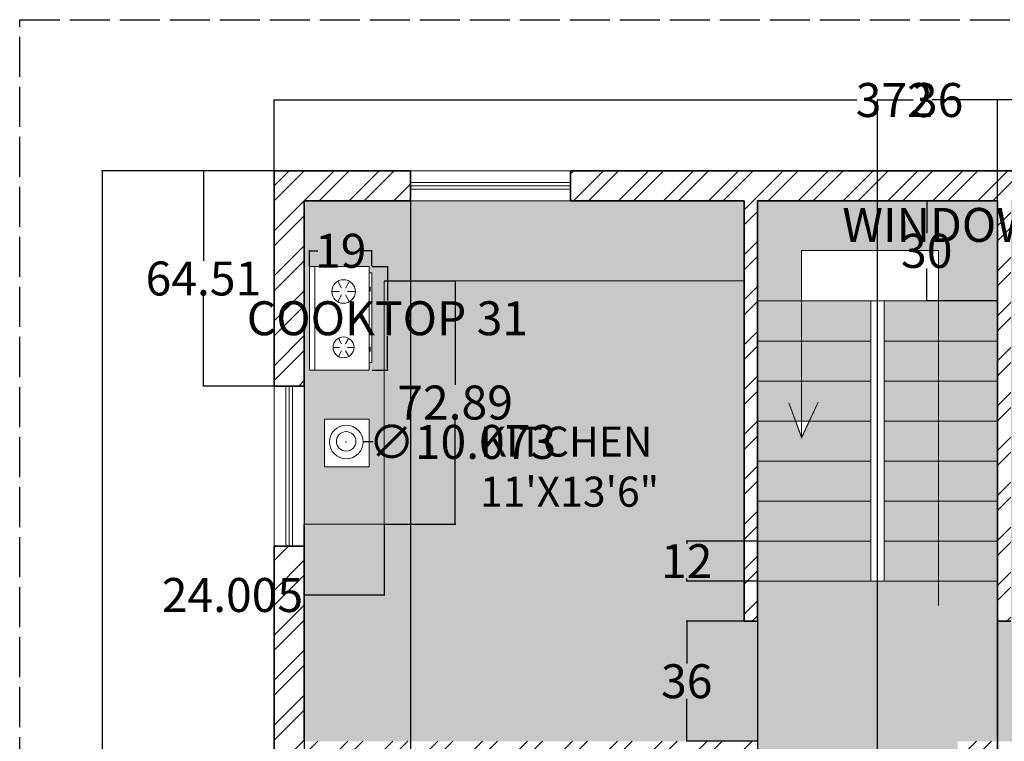
# Model space of a CAD drawing. Units: inches. Extents: x 1410 to 1959, y 5441 to 5968.
# Tile 2 of 5: x 1410 to 1705, y 5751 to 5968. Entities that reach past the tile are written whole.
import ezdxf

# ---------------------------------------------------------------- set-up
doc = ezdxf.new("R2010")
doc.units = ezdxf.units.IN
doc.linetypes.add('ACAD_ISO02W100', pattern=[15, 12, -3])
doc.layers.get('Defpoints').update_dxf_attribs({"linetype": 'ACAD_ISO02W100'})
for name, color, linetype, lineweight in [('A-ANNO-DIMS', 2, 'Continuous', 18), ('A-ANNO-SYMB', 7, 'Continuous', 18), ('A-AREA-IDEN', 7, 'Continuous', 18), ('A-EQPM', 15, 'Continuous', 15), ('A-FLOR-CABT', 15, 'Continuous', 18), ('A-FLOR-FIXT', 9, 'Continuous', 18), ('A-FLOR-STRS', 7, 'Continuous', 18), ('A-WALL', 7, 'Continuous', 35), ('A-WALL-PATT', 8, 'Continuous', 13), ('WINDOW', 160, 'Continuous', 13)]:
    doc.layers.add(name, color=color, linetype=linetype, lineweight=lineweight)
for name, color, linetype, lineweight, true_color in [('A-FLOR-CABT-PATT', 165, 'Continuous', 9, 0x5e67af), ('A-FLOR-PATT', 9, 'Continuous', 9, 0xafd9aa), ('A-FLOR-STRS-PATT', 254, 'Continuous', 9, 0xddb3d4), ('FURN3D', 229, 'Continuous', 5, 0x4a3f41)]:
    doc.layers.add(name, color=color, linetype=linetype, lineweight=lineweight, true_color=true_color)
doc.styles.get("Standard").update_dxf_attribs({"font": 'arial.ttf'})
doc.dimstyles.get("Standard").update_dxf_attribs({"dimtxt": 10.18, "dimasz": 0.18, "dimexe": 0.18, "dimexo": 0.0625, "dimgap": 0.09, "dimtad": 0, "dimtih": 1, "dimtoh": 1, "dimdec": 0, "dimzin": 0, "dimdsep": 46, "dimlunit": 3, "dimtxsty": 'Standard', "dimcen": 0.09, "dimadec": 0, "dimazin": 0, "dimtfac": 1, "dimtdec": 0, "dimtofl": 0, "dimtmove": 0, "dimatfit": 3, "dimfxl": 1, "dimtolj": 1, "dimtzin": 0, "dimarcsym": 0})

# ---------------------------------------------------------------- blocks, each defined once
blk = doc.blocks.new('A$C21540130')
at = {"layer": 'FURN3D'}
for p, q in [((1.57, 0), (1.57, 31.11)), ((9.61, 25.31), (8.63, 27.01)), ((10.79, 25.31), (11.77, 27.01)), ((9.02, 24.29, -27.54), (7.06, 24.29, -27.54)), ((11.38, 24.29, -27.54), (13.34, 24.29, -27.54)), ((9.61, 23.27), (8.63, 21.57)), ((10.79, 23.27), (11.77, 21.57)), ((9.61, 8.56), (8.43, 10.6)), ((10.79, 8.56), (11.97, 10.6)), ((9.02, 7.54), (6.67, 7.54)), ((9.61, 6.52), (8.43, 4.48)), ((10.79, 6.52), (11.97, 4.48)), ((11.38, 7.54), (13.73, 7.54))]:
    blk.add_line(p, q, dxfattribs=at)
for points in [[(0, 0), (0, 31.11), (17.9, 31.11), (17.9, 0)], [(18.68, 1.96), (18.68, 28.83), (17.9, 28.83), (17.9, 1.96)]]:
    blk.add_lwpolyline(points, close=True, dxfattribs=at)
for centre, radius in [((10.2, 24.29), 3.14), ((10.2, 7.54), 3.53)]:
    blk.add_circle(centre, radius, dxfattribs=at)
for points in [[(17.9, 24.03), (18.29, 24.03), (17.9, 25.6), (18.29, 25.6)], [(17.9, 6.05), (18.29, 6.05), (17.9, 7.62), (18.29, 7.62)]]:
    blk.add_solid(points, dxfattribs=at)
blk = doc.blocks.new('WIN-48IN')
for p, q in [((48, 9), (0, 9)), ((0, 5.5), (48, 5.5)), ((0, 4.5), (48, 4.5)), ((0, 3.5), (48, 3.5)), ((0, 0), (48, 0))]:
    blk.add_line(p, q)
blk = doc.blocks.new('*D10')
at = {"layer": 'A-ANNO-DIMS', "color": 0, "lineweight": -2, "transparency": 16777216}
for p, q in [((1769.1, 5913.3), (1769.1, 5905.99)), ((1817.1, 5913.3), (1817.1, 5905.99)), ((1769.1, 5906.17), (1768.92, 5906.17)), ((1816.92, 5906.17), (1769.28, 5906.17))]:
    blk.add_line(p, q, dxfattribs=at)
at = {"layer": 'A-ANNO-DIMS', "color": 0, "transparency": 16777216}
for points in [[(1769.28, 5906.2), (1769.28, 5906.14), (1769.1, 5906.17)], [(1816.92, 5906.2), (1816.92, 5906.14), (1817.1, 5906.17)]]:
    blk.add_solid(points, dxfattribs=at)
at = {"layer": 'Defpoints', "color": 0, "transparency": 16777216}
for p in [(1769.1, 5913.37), (1817.1, 5913.37), (1769.1, 5906.17)]:
    blk.add_point(p, dxfattribs=at)
at = {"layer": 'A-ANNO-DIMS', "color": 0, "transparency": 16777216, "insert": (1710.67, 5906.17), "char_height": 10.18, "attachment_point": 5}
blk.add_mtext('\\A1;WINDOW 48 TYP.', dxfattribs=at)
blk = doc.blocks.new('*D20')
at = {"layer": 'A-ANNO-DIMS', "color": 0, "lineweight": -2, "transparency": 16777216}
for p, q in [((1515.44, 5893.75), (1520.23, 5893.75)), ((1520.05, 5893.57), (1520.05, 5883.56)), ((1520.05, 5862.82), (1520.05, 5872.83)), ((1515.44, 5862.64), (1520.23, 5862.64))]:
    blk.add_line(p, q, dxfattribs=at)
at = {"layer": 'A-ANNO-DIMS', "color": 0, "transparency": 16777216}
for points in [[(1520.02, 5893.57), (1520.08, 5893.57), (1520.05, 5893.75)], [(1520.02, 5862.82), (1520.08, 5862.82), (1520.05, 5862.64)]]:
    blk.add_solid(points, dxfattribs=at)
at = {"layer": 'Defpoints', "color": 0, "transparency": 16777216}
for p in [(1515.38, 5893.75), (1515.38, 5862.64), (1520.05, 5862.64)]:
    blk.add_point(p, dxfattribs=at)
at = {"layer": 'A-ANNO-DIMS', "color": 0, "transparency": 16777216, "insert": (1520.05, 5878.19), "char_height": 10.18, "attachment_point": 5}
blk.add_mtext('\\A1;COOKTOP 31', dxfattribs=at)
blk = doc.blocks.new('*D21')
at = {"layer": 'A-ANNO-DIMS', "color": 0, "lineweight": -2, "transparency": 16777216}
for p, q in [((1496.7, 5893.81), (1496.7, 5898.59)), ((1496.88, 5898.41), (1499.13, 5898.41)), ((1515.2, 5898.41), (1512.95, 5898.41)), ((1515.38, 5893.81), (1515.38, 5898.59))]:
    blk.add_line(p, q, dxfattribs=at)
at = {"layer": 'A-ANNO-DIMS', "color": 0, "transparency": 16777216}
for points in [[(1496.88, 5898.44), (1496.88, 5898.38), (1496.7, 5898.41)], [(1515.2, 5898.44), (1515.2, 5898.38), (1515.38, 5898.41)]]:
    blk.add_solid(points, dxfattribs=at)
at = {"layer": 'Defpoints', "color": 0, "transparency": 16777216}
for p in [(1515.38, 5898.41), (1496.7, 5893.75), (1515.38, 5893.75)]:
    blk.add_point(p, dxfattribs=at)
at = {"layer": 'A-ANNO-DIMS', "color": 0, "transparency": 16777216, "insert": (1506.04, 5898.41), "char_height": 10.18, "attachment_point": 5}
blk.add_mtext('\\A1;19', dxfattribs=at)
blk = doc.blocks.new('*D24')
at = {"layer": 'A-ANNO-DIMS', "color": 0, "lineweight": -2, "transparency": 16777216}
for p, q in [((1486.09, 5922.43), (1486.09, 5943.8)), ((1486.27, 5943.62), (1660.81, 5943.62)), ((1857.91, 5943.62), (1683.37, 5943.62)), ((1858.09, 5922.43), (1858.09, 5943.8))]:
    blk.add_line(p, q, dxfattribs=at)
at = {"layer": 'A-ANNO-DIMS', "color": 0, "transparency": 16777216}
for points in [[(1486.27, 5943.65), (1486.27, 5943.59), (1486.09, 5943.62)], [(1857.91, 5943.65), (1857.91, 5943.59), (1858.09, 5943.62)]]:
    blk.add_solid(points, dxfattribs=at)
at = {"layer": 'Defpoints', "color": 0, "transparency": 16777216}
for p in [(1858.09, 5943.62), (1486.09, 5922.37), (1858.09, 5922.37)]:
    blk.add_point(p, dxfattribs=at)
at = {"layer": 'A-ANNO-DIMS', "color": 0, "transparency": 16777216, "insert": (1672.09, 5943.62), "char_height": 10.18, "attachment_point": 5}
blk.add_mtext('\\A1;372', dxfattribs=at)
blk = doc.blocks.new('*D25')
at = {"layer": 'A-ANNO-DIMS', "color": 0, "lineweight": -2, "transparency": 16777216}
for p, q in [((1486.03, 5922.37), (1434.27, 5922.37)), ((1434.45, 5922.19), (1434.45, 5729.66)), ((1434.45, 5526.55), (1434.45, 5719.07)), ((1703.03, 5526.37), (1434.27, 5526.37))]:
    blk.add_line(p, q, dxfattribs=at)
at = {"layer": 'A-ANNO-DIMS', "color": 0, "transparency": 16777216}
for points in [[(1434.42, 5922.19), (1434.48, 5922.19), (1434.45, 5922.37)], [(1434.42, 5526.55), (1434.48, 5526.55), (1434.45, 5526.37)]]:
    blk.add_solid(points, dxfattribs=at)
at = {"layer": 'Defpoints', "color": 0, "transparency": 16777216}
for p in [(1434.45, 5922.37), (1486.09, 5922.37), (1703.09, 5526.37)]:
    blk.add_point(p, dxfattribs=at)
at = {"layer": 'A-ANNO-DIMS', "color": 0, "transparency": 16777216, "insert": (1434.45, 5724.37), "char_height": 10.18, "attachment_point": 5}
blk.add_mtext('\\A1;396', dxfattribs=at)
blk = doc.blocks.new('*D27')
at = {"layer": 'A-ANNO-DIMS', "color": 0, "lineweight": -2, "transparency": 16777216}
for p, q in [((1495.09, 5913.3), (1495.09, 5478.87)), ((1527, 5913.3), (1527, 5478.87)), ((1495.27, 5479.05), (1526.82, 5479.05)), ((1527, 5479.05), (1527.18, 5479.05))]:
    blk.add_line(p, q, dxfattribs=at)
at = {"layer": 'A-ANNO-DIMS', "color": 0, "transparency": 16777216}
for points in [[(1495.27, 5479.08), (1495.27, 5479.02), (1495.09, 5479.05)], [(1526.82, 5479.08), (1526.82, 5479.02), (1527, 5479.05)]]:
    blk.add_solid(points, dxfattribs=at)
at = {"layer": 'Defpoints', "color": 0, "transparency": 16777216}
for p in [(1495.09, 5913.37), (1527, 5913.37), (1527, 5479.05)]:
    blk.add_point(p, dxfattribs=at)
at = {"layer": 'A-ANNO-DIMS', "color": 0, "transparency": 16777216, "insert": (1548.43, 5479.05), "char_height": 10.18, "attachment_point": 5}
blk.add_mtext('\\A1;31.905', dxfattribs=at)
blk = doc.blocks.new('*D29')
at = {"layer": 'A-ANNO-DIMS', "color": 0, "lineweight": -2, "transparency": 16777216}
for p, q in [((1486.03, 5922.37), (1464.66, 5922.36)), ((1464.84, 5922.18), (1464.85, 5895.4)), ((1464.85, 5858.03), (1464.85, 5884.82)), ((1486.04, 5857.86), (1464.67, 5857.85))]:
    blk.add_line(p, q, dxfattribs=at)
at = {"layer": 'A-ANNO-DIMS', "color": 0, "transparency": 16777216}
for points in [[(1464.87, 5922.18), (1464.81, 5922.18), (1464.84, 5922.36)], [(1464.88, 5858.03), (1464.82, 5858.03), (1464.85, 5857.85)]]:
    blk.add_solid(points, dxfattribs=at)
at = {"layer": 'Defpoints', "color": 0, "transparency": 16777216}
for p in [(1464.84, 5922.36), (1486.09, 5922.37), (1486.1, 5857.86)]:
    blk.add_point(p, dxfattribs=at)
at = {"layer": 'A-ANNO-DIMS', "color": 0, "transparency": 16777216, "insert": (1464.85, 5890.11), "char_height": 10.18, "attachment_point": 5}
blk.add_mtext('\\A1;64.51', dxfattribs=at)
blk = doc.blocks.new('*D34')
at = {"layer": 'A-ANNO-DIMS', "color": 0, "lineweight": -2, "transparency": 16777216}
for p, q in [((1631.09, 5787.3), (1631.09, 5478.87)), ((1703.09, 5787.3), (1703.09, 5478.87)), ((1631.27, 5479.05), (1659.81, 5479.05)), ((1702.91, 5479.05), (1674.38, 5479.05))]:
    blk.add_line(p, q, dxfattribs=at)
at = {"layer": 'A-ANNO-DIMS', "color": 0, "transparency": 16777216}
for points in [[(1631.27, 5479.08), (1631.27, 5479.02), (1631.09, 5479.05)], [(1702.91, 5479.08), (1702.91, 5479.02), (1703.09, 5479.05)]]:
    blk.add_solid(points, dxfattribs=at)
at = {"layer": 'Defpoints', "color": 0, "transparency": 16777216}
for p in [(1631.09, 5787.37), (1703.09, 5787.37), (1703.09, 5479.05)]:
    blk.add_point(p, dxfattribs=at)
at = {"layer": 'A-ANNO-DIMS', "color": 0, "transparency": 16777216, "insert": (1667.09, 5479.05), "char_height": 10.18, "attachment_point": 5}
blk.add_mtext('\\A1;72', dxfattribs=at)
blk = doc.blocks.new('*D35')
at = {"layer": 'A-ANNO-DIMS', "color": 0, "lineweight": -2, "transparency": 16777216}
for p, q in [((1631.03, 5787.37), (1609.66, 5787.37)), ((1609.84, 5787.19), (1609.84, 5774.66)), ((1609.84, 5751.55), (1609.84, 5764.07)), ((1631.03, 5751.37), (1609.66, 5751.37))]:
    blk.add_line(p, q, dxfattribs=at)
at = {"layer": 'A-ANNO-DIMS', "color": 0, "transparency": 16777216}
for points in [[(1609.81, 5787.19), (1609.87, 5787.19), (1609.84, 5787.37)], [(1609.81, 5751.55), (1609.87, 5751.55), (1609.84, 5751.37)]]:
    blk.add_solid(points, dxfattribs=at)
at = {"layer": 'Defpoints', "color": 0, "transparency": 16777216}
for p in [(1609.84, 5787.37), (1631.09, 5787.37), (1631.09, 5751.37)]:
    blk.add_point(p, dxfattribs=at)
at = {"layer": 'A-ANNO-DIMS', "color": 0, "transparency": 16777216, "insert": (1609.84, 5769.37), "char_height": 10.18, "attachment_point": 5}
blk.add_mtext('\\A1;36', dxfattribs=at)
blk = doc.blocks.new('*D37')
at = {"layer": 'A-ANNO-DIMS', "color": 0, "lineweight": -2, "transparency": 16777216}
for p, q in [((1667.09, 5594.43), (1667.09, 5943.8)), ((1667.27, 5943.62), (1677.72, 5943.62)), ((1702.91, 5943.62), (1692.47, 5943.62)), ((1703.09, 5558.43), (1703.09, 5943.8))]:
    blk.add_line(p, q, dxfattribs=at)
at = {"layer": 'A-ANNO-DIMS', "color": 0, "transparency": 16777216}
for points in [[(1667.27, 5943.65), (1667.27, 5943.59), (1667.09, 5943.62)], [(1702.91, 5943.65), (1702.91, 5943.59), (1703.09, 5943.62)]]:
    blk.add_solid(points, dxfattribs=at)
at = {"layer": 'Defpoints', "color": 0, "transparency": 16777216}
for p in [(1703.09, 5943.62), (1667.09, 5594.37), (1703.09, 5558.37)]:
    blk.add_point(p, dxfattribs=at)
at = {"layer": 'A-ANNO-DIMS', "color": 0, "transparency": 16777216, "insert": (1685.09, 5943.62), "char_height": 10.18, "attachment_point": 5}
blk.add_mtext('\\A1;36', dxfattribs=at)
blk = doc.blocks.new('*D49')
at = {"layer": 'A-ANNO-DIMS', "color": 0, "lineweight": -2, "transparency": 16777216}
for p, q in [((1495.09, 5816.41), (1495.09, 5795.04)), ((1519.1, 5816.41), (1519.1, 5795.04)), ((1495.09, 5795.22), (1494.91, 5795.22)), ((1518.92, 5795.22), (1495.27, 5795.22))]:
    blk.add_line(p, q, dxfattribs=at)
at = {"layer": 'A-ANNO-DIMS', "color": 0, "transparency": 16777216}
for points in [[(1495.27, 5795.25), (1495.27, 5795.19), (1495.09, 5795.22)], [(1518.92, 5795.25), (1518.92, 5795.19), (1519.1, 5795.22)]]:
    blk.add_solid(points, dxfattribs=at)
at = {"layer": 'Defpoints', "color": 0, "transparency": 16777216}
for p in [(1495.09, 5816.47), (1519.1, 5816.47), (1495.09, 5795.22)]:
    blk.add_point(p, dxfattribs=at)
at = {"layer": 'A-ANNO-DIMS', "color": 0, "transparency": 16777216, "insert": (1473.57, 5795.22), "char_height": 10.18, "attachment_point": 5}
blk.add_mtext('\\A1;24.005', dxfattribs=at)
blk = doc.blocks.new('*D50')
at = {"layer": 'A-ANNO-DIMS', "color": 0, "lineweight": -2, "transparency": 16777216}
for p, q in [((1519.16, 5889.37), (1540.53, 5889.37)), ((1540.35, 5889.19), (1540.35, 5858.21)), ((1540.35, 5816.65), (1540.35, 5847.63)), ((1519.16, 5816.47), (1540.53, 5816.47))]:
    blk.add_line(p, q, dxfattribs=at)
at = {"layer": 'A-ANNO-DIMS', "color": 0, "transparency": 16777216}
for points in [[(1540.32, 5889.19), (1540.38, 5889.19), (1540.35, 5889.37)], [(1540.32, 5816.65), (1540.38, 5816.65), (1540.35, 5816.47)]]:
    blk.add_solid(points, dxfattribs=at)
at = {"layer": 'Defpoints', "color": 0, "transparency": 16777216}
for p in [(1519.1, 5889.37), (1519.1, 5816.47), (1540.35, 5816.47)]:
    blk.add_point(p, dxfattribs=at)
at = {"layer": 'A-ANNO-DIMS', "color": 0, "transparency": 16777216, "insert": (1540.35, 5852.92), "char_height": 10.18, "attachment_point": 5}
blk.add_mtext('\\A1;72.89', dxfattribs=at)
blk = doc.blocks.new('*D51')
at = {"layer": 'A-ANNO-DIMS', "color": 0, "lineweight": -2, "transparency": 16777216}
for p, q in [((1631.03, 5811.37), (1609.66, 5811.37)), ((1609.84, 5811.19), (1609.84, 5810.57)), ((1631.03, 5799.37), (1609.66, 5799.37)), ((1609.84, 5799.55), (1609.84, 5800.17))]:
    blk.add_line(p, q, dxfattribs=at)
at = {"layer": 'A-ANNO-DIMS', "color": 0, "transparency": 16777216}
for points in [[(1609.81, 5811.19), (1609.87, 5811.19), (1609.84, 5811.37)], [(1609.81, 5799.55), (1609.87, 5799.55), (1609.84, 5799.37)]]:
    blk.add_solid(points, dxfattribs=at)
at = {"layer": 'Defpoints', "color": 0, "transparency": 16777216}
for p in [(1609.84, 5811.37), (1631.09, 5811.37), (1631.09, 5799.37)]:
    blk.add_point(p, dxfattribs=at)
at = {"layer": 'A-ANNO-DIMS', "color": 0, "transparency": 16777216, "insert": (1609.84, 5805.37), "char_height": 10.18, "attachment_point": 5}
blk.add_mtext('\\A1;12', dxfattribs=at)
blk = doc.blocks.new('*D52')
at = {"layer": 'A-ANNO-DIMS', "color": 0, "lineweight": -2, "transparency": 16777216}
for p, q in [((1703.03, 5913.37), (1681.66, 5913.37)), ((1681.84, 5913.19), (1681.84, 5903.66)), ((1681.84, 5883.55), (1681.84, 5893.07)), ((1703.03, 5883.37), (1681.66, 5883.37))]:
    blk.add_line(p, q, dxfattribs=at)
at = {"layer": 'A-ANNO-DIMS', "color": 0, "transparency": 16777216}
for points in [[(1681.81, 5913.19), (1681.87, 5913.19), (1681.84, 5913.37)], [(1681.81, 5883.55), (1681.87, 5883.55), (1681.84, 5883.37)]]:
    blk.add_solid(points, dxfattribs=at)
at = {"layer": 'Defpoints', "color": 0, "transparency": 16777216}
for p in [(1681.84, 5913.37), (1703.09, 5913.37), (1703.09, 5883.37)]:
    blk.add_point(p, dxfattribs=at)
at = {"layer": 'A-ANNO-DIMS', "color": 0, "transparency": 16777216, "insert": (1681.84, 5898.37), "char_height": 10.18, "attachment_point": 5}
blk.add_mtext('\\A1;30', dxfattribs=at)
blk = doc.blocks.new('*D61')
at = {"layer": 'A-ANNO-DIMS', "color": 0, "lineweight": -2, "transparency": 16777216}
for p, q in [((1507.61, 5841.11), (1507.79, 5841.11)), ((1507.7, 5841.02), (1507.7, 5841.2)), ((1515.76, 5841.11), (1512.91, 5841.11))]:
    blk.add_line(p, q, dxfattribs=at)
at = {"layer": 'A-ANNO-DIMS', "color": 0, "transparency": 16777216}
blk.add_solid([(1512.91, 5841.14), (1512.91, 5841.08), (1512.73, 5841.11)], dxfattribs=at)
at = {"layer": 'Defpoints', "color": 0, "transparency": 16777216}
for p in [(1502.66, 5841.11), (1512.73, 5841.11)]:
    blk.add_point(p, dxfattribs=at)
at = {"layer": 'A-ANNO-DIMS', "color": 0, "transparency": 16777216, "insert": (1542.52, 5841.11), "char_height": 10.18, "attachment_point": 5}
blk.add_mtext('\\A1;∅10.073', dxfattribs=at)

msp = doc.modelspace()

# ---------------------------------------------------------------- hatches: boundary and pattern name
at = {"layer": 'A-FLOR-CABT-PATT'}
h = msp.add_hatch(color=256, dxfattribs=at)
h.dxf.hatch_style = 1
h.paths.add_polyline_path([(1495.0981, 5857.856), (1495.0942, 5913.3659), (1526.9987, 5913.3659), (1574.9993, 5913.3659), (1627.0942, 5913.3659), (1627.0942, 5889.3659), (1519.0989, 5889.3659), (1519.0989, 5816.4745), (1495.0942, 5816.4745), (1495.0942, 5816.4792)])
h.paths.add_polyline_path([(1515.3809, 5891.786), (1515.3809, 5864.9133), (1514.5963, 5864.9133), (1514.5963, 5862.6415), (1496.6963, 5862.6415), (1496.6963, 5893.7475), (1514.5963, 5893.7475), (1514.5963, 5891.786)], flags=16)
h.paths.add_polyline_path([(1510.4271, 5886.2066, -1), (1503.3655, 5886.2066, -1)], flags=0)
h.paths.add_polyline_path([(1510.0348, 5869.4573, -1), (1503.7579, 5869.4573, -1)], flags=0)
h.paths.add_polyline_path([(1514.6117, 5847.9188), (1514.6117, 5833.6255), (1501.1483, 5833.6255), (1501.1483, 5847.9188)], flags=16)
h.paths.add_polyline_path([(1512.7347, 5841.1074, -1), (1502.6617, 5841.1074, -1)], flags=0)
h.paths.add_polyline_path([(1510.5996, 5841.2787, -1), (1504.7353, 5841.2787, -1)], flags=0)
at = {"layer": 'A-FLOR-PATT', "transparency": 33554534}
h = msp.add_hatch(color=256, dxfattribs=at)
h.dxf.hatch_style = 1
h.paths.add_polyline_path([(1849.0942, 5913.3659), (1817.1029, 5913.3659), (1769.1029, 5913.3659), (1769.1029, 5913.3659), (1707.0942, 5913.3659), (1707.0942, 5787.3659), (1703.0942, 5787.3659), (1703.0942, 5799.3659), (1631.0942, 5799.3659), (1631.0942, 5787.3659), (1627.0942, 5787.3659), (1627.0942, 5889.3659), (1519.0989, 5889.3659), (1519.0989, 5816.4745), (1495.0981, 5816.4745), (1495.0981, 5809.856), (1495.0942, 5751.3659), (1631.0942, 5751.3659), (1631.0942, 5747.3659), (1495.0942, 5747.3659), (1495.0942, 5702.5811), (1495.0984, 5654.5768), (1495.0942, 5603.3659), (1667.0942, 5603.3659), (1667.0942, 5594.3659), (1650.778, 5594.3659), (1650.778, 5558.3659), (1703.0942, 5558.3659), (1703.0942, 5594.3659), (1703.0942, 5711.3659), (1707.0942, 5711.3659), (1707.0942, 5535.3659), (1754.5413, 5535.3659), (1802.541, 5535.3658), (1802.5413, 5535.3658), (1802.5413, 5535.3659), (1849.0942, 5535.3659), (1849.0942, 5651.3659), (1743.0942, 5651.3659), (1743.0942, 5655.3659), (1849.0942, 5655.3659), (1849.0942, 5665.4579), (1849.0942, 5689.4579), (1849.0942, 5699.3659), (1801.0942, 5699.3659), (1801.0942, 5685.3659), (1797.0942, 5685.3659), (1797.0942, 5699.3659), (1783.0942, 5699.3659), (1783.0942, 5703.3659), (1849.0942, 5703.3659), (1849.0942, 5716.9764), (1849.123, 5716.9764), (1849.123, 5740.9654), (1849.0942, 5740.9654), (1849.0942, 5747.3659), (1753.0942, 5747.3659), (1753.0942, 5699.3659), (1749.0942, 5699.3659), (1749.0942, 5747.3659), (1707.0942, 5747.3659), (1691.0942, 5747.3659), (1691.0942, 5751.3659), (1707.0942, 5751.3659), (1849.0942, 5751.3659)])
h.paths.add_polyline_path([(1533.4842, 5711.1518), (1533.4842, 5637.9201), (1534.7464, 5637.9201), (1534.7464, 5640.1099, -0.41421356), (1536.9363, 5642.2998), (1558.8347, 5642.2998, -0.41421356), (1561.0246, 5640.1099), (1561.0246, 5637.9201), (1563.2144, 5637.9201, -0.41421356), (1565.4042, 5635.7302), (1565.4042, 5609.4519, -0.41421356), (1563.2144, 5607.2621), (1532.5566, 5607.2621, -0.41421356), (1530.3668, 5609.4519), (1530.3668, 5635.4862), (1529.1045, 5635.4862), (1529.1045, 5633.2964, -0.41421356), (1526.9147, 5631.1065), (1500.6363, 5631.1065, -0.41421356), (1498.4465, 5633.2964), (1498.4465, 5715.5315, -0.41421356), (1500.6363, 5717.7213), (1526.9147, 5717.7213, -0.41421356), (1529.1045, 5715.5315), (1529.1045, 5713.3417), (1531.2944, 5713.3417, -0.41421356)], flags=16)
h.paths.add_polyline_path([(1771.0631, 5793.9619), (1771.0631, 5835.0118), (1771.0631, 5856.9619, -0.41421356), (1771.9631, 5857.8619), (1842.1181, 5857.8619, -0.41421356), (1843.0181, 5856.9619), (1843.0181, 5857.8619), (1846.6631, 5857.8619), (1846.6631, 5793.0619), (1843.0181, 5793.0619), (1828.4381, 5793.0619), (1771.9631, 5793.0619, -0.41421356)], flags=16)
h.paths.add_polyline_path([(1771.0631, 5805.9671, 0.25346465), (1781.0166, 5803.0153, 0.25379956), (1783.9781, 5793.0522)], flags=16)
h.paths.add_polyline_path([(1746.3058, 5612.0795), (1768.2559, 5612.0795), (1809.3058, 5612.0795, -0.41421356), (1810.2058, 5611.1795), (1810.2058, 5554.7045), (1810.2058, 5540.1245), (1810.2058, 5536.4795), (1745.4058, 5536.4795), (1745.4058, 5540.1245), (1746.3058, 5540.1245, -0.41421356), (1745.4058, 5541.0245), (1745.4058, 5611.1795, -0.41421356)], flags=16)
h.paths.add_polyline_path([(1819.5646, 5793.1537), (1819.5646, 5793.8054, 0.05271893), (1808.0815, 5849.0458, 0.29223153), (1819.5646, 5857.6981), (1828.4381, 5857.6981), (1828.4381, 5857.0464), (1828.4381, 5847.601, -0.06332793), (1838.1593, 5837.9401, -0.38046479), (1838.3062, 5835.5217, -0.02593615), (1834.5989, 5831.2824, -0.02509022), (1838.1593, 5827.1584, -0.38046478), (1838.3062, 5824.74, -0.05941785), (1829.2061, 5815.646, -0.11763956), (1828.4381, 5815.2914), (1828.4381, 5793.1537)], flags=0)
h.paths.add_polyline_path([(1819.5646, 5793.1537), (1819.5646, 5822.5662, -0.01603557), (1817.3363, 5825.2436, -0.4295765), (1817.4052, 5827.8865, -0.01537126), (1819.5646, 5830.4335), (1819.5646, 5833.3479, -0.01603557), (1817.3363, 5836.0254, -0.48413611), (1817.6682, 5838.8652, 0.00079305), (1817.0318, 5838.199, 0.26524804), (1817.0526, 5836.3926, 0.02736634), (1820.9176, 5831.8795, 0.02734261), (1817.0221, 5827.3996, 0.26229506), (1817.0526, 5825.6108, 0.06555279), (1827.0712, 5815.5721), (1827.0712, 5793.1537)], flags=0)
h.paths.add_polyline_path([(1830.4631, 5775.9619), (1830.4631, 5792.1619), (1846.6631, 5792.1619), (1846.6631, 5775.9619)], flags=16)
h.paths.add_polyline_path([(1831.3631, 5776.8619), (1831.3631, 5791.2619), (1845.7631, 5791.2619), (1845.7631, 5776.8619)], flags=0)
h.paths.add_polyline_path([(1836.6983, 5784.1006, -1), (1843.9547, 5784.1006, -1)], flags=0)
h.paths.add_polyline_path([(1819.2615, 5682.5311, -0.25820517), (1830.2865, 5687.0962, -0.1716359), (1835.799, 5683.9093), (1838.1615, 5683.9093), (1838.1615, 5688.0436, -0.41421356), (1839.1458, 5689.028), (1845.4458, 5689.028, -0.41421356), (1846.4302, 5688.0436), (1846.4302, 5671.8999, -0.41421356), (1845.4458, 5670.9155), (1839.1458, 5670.9155, -0.41421356), (1838.1615, 5671.8999), (1838.1615, 5676.0343), (1835.799, 5676.0343, -0.1716359), (1830.2865, 5672.8474, -0.25820517), (1819.2615, 5677.4124)], flags=16)
h.paths.add_polyline_path([(1820.8043, 5682.5681, -0.21038447), (1830.2865, 5685.5212, -0.1716359), (1835.799, 5682.3343), (1835.799, 5677.6093, -0.1716359), (1830.2865, 5674.4224, -0.21038447), (1820.8043, 5677.3755)], flags=0)
h.paths.add_polyline_path([(1842.0614, 5784.0231), (1841.8811, 5784.0231, -0.54460611), (1839.6163, 5782.7155), (1839.5262, 5782.5594, 0.54796211)], flags=0)
h.paths.add_polyline_path([(1840.3713, 5784.1781), (1840.3265, 5784.2556), (1840.2818, 5784.1781)], flags=0)
h.paths.add_polyline_path([(1830.4631, 5858.7619), (1830.4631, 5874.9619), (1846.6631, 5874.9619), (1846.6631, 5858.7619)], flags=16)
h.paths.add_polyline_path([(1831.3631, 5859.6619), (1831.3631, 5874.0619), (1845.7631, 5874.0619), (1845.7631, 5859.6619)], flags=0)
h.paths.add_polyline_path([(1755.6206, 5556.6903, -0.00089292), (1756.3396, 5557.4382), (1745.5695, 5557.4382), (1745.5695, 5554.7045), (1746.2212, 5554.7045), (1755.5673, 5554.7045, -0.38881883)], flags=0)
h.paths.add_polyline_path([(1810.114, 5563.578), (1810.114, 5554.7045), (1809.4622, 5554.7045), (1787.9762, 5554.7045, -0.11778508), (1787.6251, 5553.9338, -0.05941785), (1778.5249, 5544.8398, -0.37985907), (1776.1092, 5544.9833, -0.02509022), (1771.9852, 5548.5437, 0.03343123), (1776.8399, 5553.9365, 0.30845915), (1776.98, 5555.985, 0.04782679), (1769.9197, 5563.578), (1772.8341, 5563.578, -0.01537126), (1775.3811, 5565.7373, -0.4295765), (1778.024, 5565.8063, -0.01603557), (1780.7015, 5563.578)], flags=0)
h.paths.add_polyline_path([(1728.3058, 5552.6795), (1744.5058, 5552.6795), (1744.5058, 5536.4795), (1728.3058, 5536.4795)], flags=16)
h.paths.add_polyline_path([(1810.2058, 5599.1742, 0.25346465), (1800.2523, 5602.126, 0.25379956), (1797.2908, 5612.0892)], flags=16)
h.paths.add_polyline_path([(1843.9547, 5866.8231, -1), (1836.6983, 5866.8231, -1)], flags=0)
h.paths.add_polyline_path([(1729.2058, 5551.7795), (1743.6058, 5551.7795), (1743.6058, 5537.3795), (1729.2058, 5537.3795)], flags=0)
h.paths.add_polyline_path([(1839.4821, 5865.5155), (1840.237, 5866.8231), (1839.4821, 5868.1307, 0.25464572), (1838.77, 5866.8231, 0.25464572)], flags=0)
h.paths.add_polyline_path([(1842.0614, 5866.7456), (1840.3713, 5866.7456), (1839.5262, 5865.2819, 0.54796211)], flags=0)
h.paths.add_polyline_path([(1732.8163, 5542.8161, -1), (1740.0727, 5542.8161, -1)], flags=0)
h.paths.add_polyline_path([(1737.8296, 5543.5262), (1736.522, 5542.7713), (1736.522, 5541.2615, 0.39969799), (1738.001, 5542.8161, 0.11900365)], flags=0)
h.paths.add_polyline_path([(1738.1811, 5542.8161, -1), (1734.7079, 5542.8161, -1)], flags=0)
h.paths.add_polyline_path([(1736.4445, 5542.9056), (1736.367, 5542.9503), (1736.367, 5542.8608)], flags=0)
h.paths.add_polyline_path([(1811.1058, 5552.6795), (1827.3058, 5552.6795), (1827.3058, 5536.4795), (1811.1058, 5536.4795)], flags=16)
h.paths.add_polyline_path([(1812.0058, 5551.7795), (1826.4058, 5551.7795), (1826.4058, 5537.3795), (1812.0058, 5537.3795)], flags=0)
h.paths.add_polyline_path([(1815.5388, 5542.8161, -1), (1822.7952, 5542.8161, -1)], flags=0)
h.paths.add_polyline_path([(1820.5521, 5543.5262), (1819.2445, 5542.7713), (1819.2445, 5541.2615, 0.39969799), (1820.7235, 5542.8161, 0.11900365)], flags=0)
h.paths.add_polyline_path([(1820.9036, 5542.8161, -1), (1817.4304, 5542.8161, -1)], flags=0)
h.paths.add_polyline_path([(1819.167, 5542.9056), (1819.0895, 5542.9503), (1819.0895, 5542.8608)], flags=0)
h.paths.add_polyline_path([(1707.0264, 5710.8395), (1750.0905, 5710.8395), (1750.0905, 5723.2037), (1707.0264, 5723.2037)], flags=25)
h.paths.add_polyline_path([(1786.4108, 5658.162), (1818.7518, 5658.162), (1818.7518, 5680.5262), (1786.4108, 5680.5262)], flags=24)
h.paths.add_polyline_path([(1787.0609, 5715.7465), (1838.4906, 5715.7465), (1838.4906, 5738.1353), (1787.0609, 5738.1353)], flags=24)
h.paths.add_polyline_path([(1743.8116, 5616.0244), (1813.7243, 5616.0244), (1813.7243, 5649.6076), (1743.8116, 5649.6076)], flags=24)
h.paths.add_polyline_path([(1719.2569, 5867.7974), (1789.1696, 5867.7974), (1789.1696, 5901.3806), (1719.2569, 5901.3806)], flags=24)
h.paths.add_polyline_path([(1562.3198, 5677.907), (1619.4324, 5677.907), (1619.4324, 5711.4902), (1562.3198, 5711.4902)], flags=24)
h.paths.add_polyline_path([(1544.1706, 5816.5955), (1604.3036, 5816.5955), (1604.3036, 5850.1787), (1544.1706, 5850.1787)], flags=24)
at = {"layer": 'A-FLOR-STRS-PATT'}
h = msp.add_hatch(color=256, dxfattribs=at)
h.dxf.hatch_style = 1
h.paths.add_polyline_path([(1665.0942, 5835.3659), (1631.0942, 5835.3659), (1631.0942, 5823.3659), (1665.0942, 5823.3659)])
h.paths.add_polyline_path([(1665.0942, 5823.3659), (1631.0942, 5823.3659), (1631.0942, 5811.3659), (1665.0942, 5811.3659)])
h.paths.add_polyline_path([(1665.0942, 5811.3659), (1631.0942, 5811.3659), (1631.0942, 5799.3659), (1665.0942, 5799.3659)])
h.paths.add_polyline_path([(1665.0942, 5847.3659), (1646.6169, 5847.3659), (1644.2286, 5842.2744), (1644.2286, 5842.467), (1642.4245, 5847.3659), (1631.0942, 5847.3659), (1631.0942, 5835.3659), (1665.0942, 5835.3659)])
h.paths.add_polyline_path([(1665.0942, 5859.3659), (1644.2286, 5859.3659), (1644.2286, 5847.3659), (1646.5881, 5847.3659), (1649.2828, 5853.0491), (1646.6169, 5847.3659), (1665.0942, 5847.3659)])
h.paths.add_polyline_path([(1640.421, 5852.8062), (1642.4737, 5847.3659), (1644.2286, 5847.3659), (1644.2286, 5859.3659), (1631.0942, 5859.3659), (1631.0942, 5847.3659), (1642.4245, 5847.3659)])
h.paths.add_polyline_path([(1644.2286, 5871.3659), (1631.0942, 5871.3659), (1631.0942, 5859.3659), (1644.2286, 5859.3659)])
h.paths.add_polyline_path([(1665.0942, 5871.3659), (1644.2286, 5871.3659), (1644.2286, 5859.3659), (1665.0942, 5859.3659)])
h.paths.add_polyline_path([(1665.0942, 5883.3659), (1644.2286, 5883.3659), (1644.2286, 5871.3659), (1665.0942, 5871.3659)])
h.paths.add_polyline_path([(1644.2286, 5883.3659), (1631.0942, 5883.3659), (1631.0942, 5871.3659), (1644.2286, 5871.3659)])
h.paths.add_polyline_path([(1685.3367, 5883.3659), (1669.0942, 5883.3659), (1669.0942, 5871.3659), (1685.3367, 5871.3659)])
h.paths.add_polyline_path([(1703.0942, 5883.3659), (1685.3367, 5883.3659), (1685.3367, 5871.3659), (1703.0942, 5871.3659)])
h.paths.add_polyline_path([(1685.3367, 5871.3659), (1669.0942, 5871.3659), (1669.0942, 5859.3659), (1685.3367, 5859.3659)])
h.paths.add_polyline_path([(1703.0942, 5871.3659), (1685.3367, 5871.3659), (1685.3367, 5859.3659), (1703.0942, 5859.3659)])
h.paths.add_polyline_path([(1685.3367, 5859.3659), (1669.0942, 5859.3659), (1669.0942, 5847.3659), (1685.3367, 5847.3659)])
h.paths.add_polyline_path([(1703.0942, 5859.3659), (1685.3367, 5859.3659), (1685.3367, 5847.3659), (1703.0942, 5847.3659)])
h.paths.add_polyline_path([(1685.3367, 5847.3659), (1669.0942, 5847.3659), (1669.0942, 5835.3659), (1685.3367, 5835.3659)])
h.paths.add_polyline_path([(1703.0942, 5847.3659), (1685.3367, 5847.3659), (1685.3367, 5835.3659), (1703.0942, 5835.3659)])
h.paths.add_polyline_path([(1685.3367, 5835.3659), (1669.0942, 5835.3659), (1669.0942, 5823.3659), (1685.3367, 5823.3659)])
h.paths.add_polyline_path([(1703.0942, 5835.3659), (1685.3367, 5835.3659), (1685.3367, 5823.3659), (1703.0942, 5823.3659)])
h.paths.add_polyline_path([(1685.3367, 5823.3659), (1669.0942, 5823.3659), (1669.0942, 5811.3659), (1685.3367, 5811.3659)])
h.paths.add_polyline_path([(1703.0942, 5823.3659), (1685.3367, 5823.3659), (1685.3367, 5811.3659), (1703.0942, 5811.3659)])
h.paths.add_polyline_path([(1685.3367, 5811.3659), (1669.0942, 5811.3659), (1669.0942, 5799.3659), (1685.3367, 5799.3659)])
h.paths.add_polyline_path([(1703.0942, 5811.3659), (1685.3367, 5811.3659), (1685.3367, 5799.3659), (1703.0942, 5799.3659)])
h.paths.add_polyline_path([(1703.0942, 5913.3659), (1631.0942, 5913.3659), (1631.0942, 5883.3659), (1644.2286, 5883.3659), (1644.2286, 5898.5051), (1685.3367, 5898.5051), (1685.3367, 5883.3659), (1703.0942, 5883.3659)])
at = {"layer": 'A-WALL-PATT'}
h = msp.add_hatch(dxfattribs=at)
h.set_pattern_fill('ANSI32', color=256)
h.paths.add_polyline_path([(1526.9987, 5922.3659), (1486.0942, 5922.3659), (1486.0942, 5857.8561), (1495.0942, 5857.8561), (1495.0942, 5913.3659), (1526.9987, 5913.3659)])
h.paths.add_polyline_path([(1769.1029, 5922.3659), (1574.9987, 5922.3659), (1574.9987, 5913.3659), (1574.9993, 5913.3659), (1627.0942, 5913.3659), (1627.0942, 5787.3659), (1631.0942, 5787.3659), (1631.0942, 5913.3659), (1703.0942, 5913.3659), (1703.0942, 5787.3659), (1707.0942, 5787.3659), (1707.0942, 5913.3659), (1769.1029, 5913.3659)])
h.paths.add_polyline_path([(1858.0942, 5922.3659), (1817.1029, 5922.3659), (1817.1029, 5913.3659), (1849.0942, 5913.3659), (1849.0942, 5751.3659), (1707.0942, 5751.3659), (1691.0942, 5751.3659), (1691.0942, 5747.3659), (1707.0942, 5747.3659), (1849.0942, 5747.3659), (1849.0942, 5740.9764), (1858.0942, 5740.9764)])
h.paths.add_polyline_path([(1495.0942, 5809.8561), (1486.0981, 5809.8561), (1486.0981, 5809.856), (1486.0942, 5702.5811), (1495.0942, 5702.5811), (1495.0942, 5747.3659), (1631.0942, 5747.3659), (1631.0942, 5751.3659), (1495.0942, 5751.3659)])
h.paths.add_polyline_path([(1495.0942, 5654.5811), (1486.0984, 5654.5811), (1486.0984, 5654.5768), (1486.0942, 5594.3659), (1667.0942, 5594.3659), (1667.0942, 5603.3659), (1495.0942, 5603.3659)])
h.paths.add_polyline_path([(1858.0942, 5665.4579), (1849.0942, 5665.4579), (1849.0942, 5655.3659), (1743.0942, 5655.3659), (1743.0942, 5651.3659), (1849.0942, 5651.3659), (1849.0942, 5535.3659), (1802.5413, 5535.3659), (1802.5413, 5526.3659), (1858.0942, 5526.3659)])
h.paths.add_polyline_path([(1858.0942, 5716.9654), (1849.0942, 5716.9654), (1849.0942, 5703.3659), (1783.0942, 5703.3659), (1783.0942, 5699.3659), (1797.0942, 5699.3659), (1797.0942, 5685.3659), (1801.0942, 5685.3659), (1801.0942, 5699.3659), (1849.0942, 5699.3659), (1849.0942, 5689.4579), (1858.0942, 5689.4579)])
h.paths.add_polyline_path([(1753.0942, 5747.3659), (1749.0942, 5747.3659), (1749.0942, 5699.3659), (1753.0942, 5699.3659)])
h.paths.add_polyline_path([(1707.0942, 5711.3659), (1703.0942, 5711.3659), (1703.0942, 5594.3659), (1703.0942, 5526.3659), (1754.5413, 5526.3659), (1754.5413, 5535.3658), (1754.541, 5535.3658), (1707.0942, 5535.3659)])

# ---------------------------------------------------------------- linework, layer by layer
at = {"layer": 'A-ANNO-SYMB'}
for p, q in [((1685.3367, 5898.5051), (1644.2286, 5898.5051)), ((1644.2286, 5898.5051), (1644.2286, 5842.2744)), ((1685.3367, 5792.1045), (1685.3367, 5898.5051)), ((1644.2446, 5842.4235), (1640.421, 5852.8062)), ((1640.421, 5852.8062), (1644.2446, 5842.6727)), ((1644.2286, 5842.2744), (1649.2828, 5853.0491)), ((1649.2828, 5853.0491), (1644.2446, 5842.4235))]:
    msp.add_line(p, q, dxfattribs=at)
at = {"layer": 'A-FLOR-CABT'}
for p, q in [((1519.0989, 5889.3659), (1519.0989, 5816.4745)), ((1519.0989, 5889.3659), (1627.0942, 5889.3659)), ((1495.0942, 5816.4745), (1519.0989, 5816.4745))]:
    msp.add_line(p, q, dxfattribs=at)
at = {"layer": 'A-FLOR-FIXT'}
msp.add_lwpolyline([(1501.1483, 5847.9188), (1514.6117, 5847.9188), (1514.6117, 5833.6255), (1501.1483, 5833.6255)], close=True, dxfattribs=at)
for centre, radius in [((1507.6982, 5841.1074), 5.0365), ((1507.6674, 5841.2787), 2.9321)]:
    msp.add_circle(centre, radius, dxfattribs=at)
at = {"layer": 'A-FLOR-STRS'}
for p, q in [((1631.0942, 5883.3659), (1703.0942, 5883.3659)), ((1665.0942, 5883.3659), (1665.0942, 5799.3659)), ((1669.0942, 5883.3659), (1669.0942, 5799.3659)), ((1631.0942, 5871.3659), (1665.0942, 5871.3659)), ((1669.0942, 5871.3659), (1703.0942, 5871.3659)), ((1631.0942, 5859.3659), (1665.0942, 5859.3659)), ((1669.0942, 5859.3659), (1703.0942, 5859.3659)), ((1631.0942, 5847.3659), (1665.0942, 5847.3659)), ((1669.0942, 5847.3659), (1703.0942, 5847.3659)), ((1631.0942, 5835.3659), (1665.0942, 5835.3659)), ((1669.0942, 5835.3659), (1703.0942, 5835.3659)), ((1631.0942, 5823.3659), (1665.0942, 5823.3659)), ((1669.0942, 5823.3659), (1703.0942, 5823.3659)), ((1631.0942, 5811.3659), (1665.0942, 5811.3659)), ((1669.0942, 5811.3659), (1703.0942, 5811.3659)), ((1631.0942, 5799.3659), (1703.0942, 5799.3659))]:
    msp.add_line(p, q, dxfattribs=at)
at = {"layer": 'A-WALL'}
for p, q in [((1486.0942, 5922.3659), (1526.9987, 5922.3659)), ((1486.0942, 5857.8561), (1486.0942, 5922.3659)), ((1526.9987, 5913.3659), (1526.9987, 5922.3659)), ((1574.9987, 5913.3659), (1574.9987, 5922.3659)), ((1574.9987, 5922.3659), (1769.1029, 5922.3659)), ((1495.0942, 5913.3659), (1526.9987, 5913.3659)), ((1495.0942, 5857.8561), (1495.0942, 5913.3659)), ((1574.9987, 5913.3659), (1627.0942, 5913.3659)), ((1627.0942, 5787.3659), (1627.0942, 5913.3659)), ((1631.0942, 5913.3659), (1703.0942, 5913.3659)), ((1631.0942, 5787.3659), (1631.0942, 5913.3659)), ((1703.0942, 5913.3659), (1703.0942, 5787.3659)), ((1495.0942, 5857.8561), (1486.0942, 5857.8561)), ((1495.0942, 5751.3706), (1495.0942, 5816.4792)), ((1495.0942, 5809.8561), (1486.0942, 5809.8561)), ((1486.0942, 5702.5811), (1486.0942, 5809.8561)), ((1627.0942, 5787.3659), (1631.0942, 5787.3659)), ((1703.0942, 5787.3659), (1707.0942, 5787.3659))]:
    msp.add_line(p, q, dxfattribs=at)
at = {"layer": 'Defpoints'}
msp.add_lwpolyline([(1409.7428, 5967.6887), (1920.4745, 5967.6887), (1920.4745, 5440.571), (1409.7428, 5440.571)], close=True, dxfattribs=at)

# ---------------------------------------------------------------- block references
at = {"layer": 'A-EQPM', "xscale": -1, "rotation": 180}
msp.add_blockref('A$C21540130', (1496.6964, 5893.7474), dxfattribs=at)
at = {"layer": 'WINDOW'}
msp.add_blockref('WIN-48IN', (1526.9993, 5913.3659), dxfattribs=at)
at = {"layer": 'WINDOW', "rotation": 269.9999999999973}
msp.add_blockref('WIN-48IN', (1486.0981, 5857.856), dxfattribs=at)

# ---------------------------------------------------------------- texts
at = {"layer": 'A-AREA-IDEN', "insert": (1547.7897, 5845.7002), "char_height": 9, "attachment_point": 1}
msp.add_mtext_dynamic_manual_height_columns('KITCHEN\\P11\'X13\'6"', width=124.909089, gutter_width=12.5, heights=[0], dxfattribs=at)

# ---------------------------------------------------------------- dimensions: what is measured, and where the dimension line sits
at = {"layer": 'A-ANNO-DIMS'}
for base, p1, p2, override, picture, middle in [((1858.0942, 5943.6159), (1486.0942, 5922.3659), (1858.0942, 5922.3659), {"dimdec": 0, "dimlfac": 1, "dimrnd": 0, "dimzin": 0, "dimdsep": 46, "dimlunit": 2}, '*D24', (1672.0942, 5943.6159)), ((1703.0942, 5943.6159), (1667.0942, 5594.3659), (1703.0942, 5558.3659), {"dimdec": 0, "dimlfac": 1, "dimrnd": 0, "dimzin": 0, "dimdsep": 46, "dimlunit": 2}, '*D37', (1685.0942, 5943.6159)), ((1526.9993, 5479.0498), (1495.0942, 5913.3659), (1526.9993, 5913.3659), {"dimdec": 3, "dimlfac": 1, "dimrnd": 0, "dimzin": 0, "dimdsep": 46, "dimlunit": 2}, '*D27', (1548.4348, 5479.0498)), ((1515.3809, 5898.4134), (1496.6963, 5893.7475), (1515.3809, 5893.7475), {"dimdec": 0, "dimlfac": 1, "dimrnd": 0, "dimzin": 0, "dimdsep": 46, "dimlunit": 2}, '*D21', (1506.0386, 5898.4134)), ((1703.0942, 5479.0498), (1631.0942, 5787.3659), (1703.0942, 5787.3659), {"dimdec": 0, "dimlfac": 1, "dimrnd": 0, "dimzin": 0, "dimdsep": 46, "dimlunit": 2}, '*D34', (1667.0942, 5479.0498))]:
    dim = msp.add_linear_dim(base=base, p1=p1, p2=p2, dimstyle='Standard', override=override, dxfattribs=at)
    dim.commit()
    dim.dimension.update_dxf_attribs({"geometry": picture, "text_midpoint": middle})
for base, p1, p2, angle, text, picture, middle in [((1769.1029, 5906.1659), (1817.1029, 5913.3659), (1769.1029, 5913.3659), 180, 'WINDOW <> TYP.', '*D10', (1710.6729, 5906.1659)), ((1520.0468, 5862.6415), (1515.3809, 5893.7475), (1515.3809, 5862.6415), 270, 'COOKTOP <>', '*D20', (1520.0468, 5878.1945))]:
    dim = msp.add_linear_dim(base=base, p1=p1, p2=p2, angle=angle, text=text, dimstyle='Standard', override={"dimdec": 0, "dimlfac": 1, "dimrnd": 0, "dimzin": 0, "dimdsep": 46, "dimlunit": 2}, dxfattribs=at)
    dim.commit()
    dim.dimension.update_dxf_attribs({"geometry": picture, "text_midpoint": middle})
for base, p1, p2, angle, override, picture, middle in [((1434.453, 5922.3659), (1703.0942, 5526.3659), (1486.0942, 5922.3659), 90, {"dimdec": 0, "dimlfac": 1, "dimrnd": 0, "dimzin": 0, "dimdsep": 46, "dimlunit": 2}, '*D25', (1434.453, 5724.3659)), ((1464.8442, 5922.3646), (1486.0981, 5857.856), (1486.0942, 5922.3659), 90.003428, {"dimdec": 2, "dimlfac": 1, "dimrnd": 0, "dimzin": 0, "dimdsep": 46, "dimlunit": 2}, '*D29', (1464.8462, 5890.1097)), ((1681.8442, 5913.3659), (1703.0942, 5883.3659), (1703.0942, 5913.3659), 90, {"dimdec": 0, "dimlfac": 1, "dimrnd": 0, "dimzin": 0, "dimdsep": 46, "dimlunit": 2}, '*D52', (1681.8442, 5898.3659)), ((1540.3489, 5816.4745), (1519.0989, 5889.3659), (1519.0989, 5816.4745), 270, {"dimdec": 2, "dimlfac": 1, "dimrnd": 0, "dimzin": 0, "dimdsep": 46, "dimlunit": 2}, '*D50', (1540.3489, 5852.9202)), ((1495.0942, 5795.2245), (1519.0989, 5816.4745), (1495.0942, 5816.4745), 180, {"dimdec": 3, "dimlfac": 1, "dimrnd": 0, "dimzin": 0, "dimdsep": 46, "dimlunit": 2}, '*D49', (1473.5684, 5795.2245)), ((1609.8442, 5811.3659), (1631.0942, 5799.3659), (1631.0942, 5811.3659), 90, {"dimdec": 0, "dimlfac": 1, "dimrnd": 0, "dimzin": 0, "dimdsep": 46, "dimlunit": 2}, '*D51', (1609.8442, 5805.3659)), ((1609.8442, 5787.3659), (1631.0942, 5751.3659), (1631.0942, 5787.3659), 90, {"dimdec": 0, "dimlfac": 1, "dimrnd": 0, "dimzin": 0, "dimdsep": 46, "dimlunit": 2}, '*D35', (1609.8442, 5769.3659))]:
    dim = msp.add_linear_dim(base=base, p1=p1, p2=p2, angle=angle, dimstyle='Standard', override=override, dxfattribs=at)
    dim.commit()
    dim.dimension.update_dxf_attribs({"geometry": picture, "text_midpoint": middle})
dim = msp.add_diameter_dim_2p(p1=(1502.6617, 5841.1079), p2=(1512.7347, 5841.107), dimstyle='Standard', override={"dimdec": 3, "dimlfac": 1, "dimrnd": 0, "dimzin": 0, "dimdsep": 46, "dimlunit": 2}, dxfattribs=at)
dim.commit()
dim.dimension.update_dxf_attribs({"geometry": '*D61', "text_midpoint": (1515.7566, 5841.1067), "dimtype": 163})

doc.saveas('drawing.dxf')
